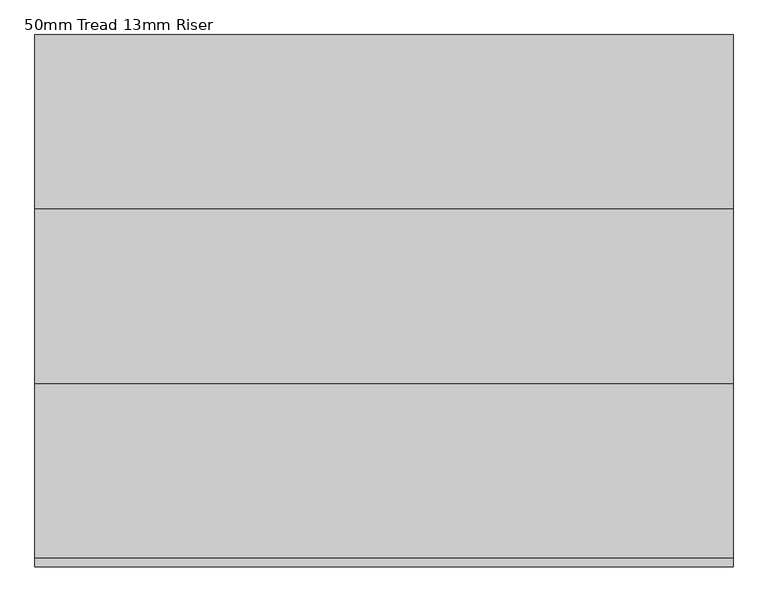
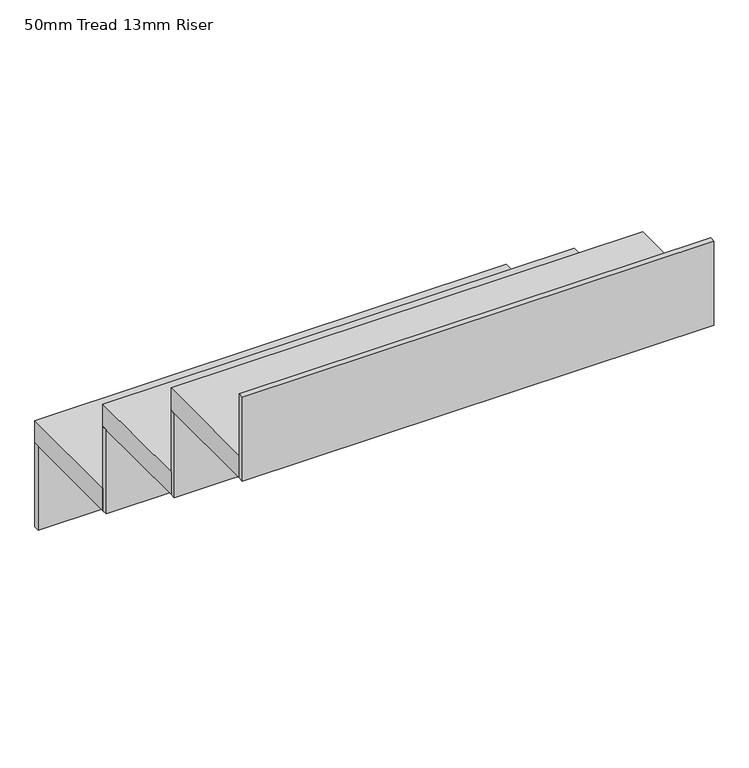
"""IFC4 building model written with IfcOpenShell, lengths in millimetres: stair flight geometry, 50mm Tread 13mm Riser."""

from ifc_helpers import new_model, si_unit, frame, origin, place, context, project, spatial, polyline, outline, extrude, source, transform, mapped, element, save


def stair_flight_50mm_tread_13mm_riser_bd8d9b2e(model_context):
    return source(origin(), model_context, "Body", "SweptSolid", [
        extrude(outline(polyline([(-10477.6052721, -2511.0618509), (-10477.6052721, -2498.5618509), (-9477.5794909, -2498.5618509), (-9477.5794909, -2511.0618509), (-10477.6052721, -2511.0618509)])), frame((0.0, 0.0, 7668.6117647), z_axis=(0.0, 0.0, 1.0), x_axis=(1.0, 0.0, 0.0)), (0.0, 0.0, 1.0), 188.2588235),
        extrude(outline(polyline([(-9477.5794909, -2748.5618509), (-10477.6052721, -2748.5618509), (-10477.6052721, -2498.5618509), (-9477.5794909, -2498.5618509), (-9477.5794909, -2748.5618509)])), frame((0.0, 0.0, 7856.8705882), z_axis=(0.0, 0.0, 1.0), x_axis=(1.0, 0.0, 0.0)), (0.0, 0.0, 1.0), 50.0),
        extrude(outline(polyline([(-10477.6052721, -2761.0618509), (-10477.6052721, -2748.5618509), (-9477.5794909, -2748.5618509), (-9477.5794909, -2761.0618509), (-10477.6052721, -2761.0618509)])), frame((0.0, 0.0, 7856.8705882), z_axis=(0.0, 0.0, 1.0), x_axis=(1.0, 0.0, 0.0)), (0.0, 0.0, 1.0), 188.2588235),
        extrude(outline(polyline([(-9477.5794909, -2998.5618509), (-10477.6052721, -2998.5618509), (-10477.6052721, -2748.5618509), (-9477.5794909, -2748.5618509), (-9477.5794909, -2998.5618509)])), frame((0.0, 0.0, 8045.1294118), z_axis=(0.0, 0.0, 1.0), x_axis=(1.0, 0.0, 0.0)), (0.0, 0.0, 1.0), 50.0),
        extrude(outline(polyline([(-10477.6052721, -3011.0618509), (-10477.6052721, -2998.5618509), (-9477.5794909, -2998.5618509), (-9477.5794909, -3011.0618509), (-10477.6052721, -3011.0618509)])), frame((0.0, 0.0, 8045.1294118), z_axis=(0.0, 0.0, 1.0), x_axis=(1.0, 0.0, 0.0)), (0.0, 0.0, 1.0), 188.2588235),
        extrude(outline(polyline([(-10477.6052721, -3261.0618509), (-10477.6052721, -3248.5618509), (-9477.5794909, -3248.5618509), (-9477.5794909, -3261.0618509), (-10477.6052721, -3261.0618509)])), frame((0.0, 0.0, 8233.3882353), z_axis=(0.0, 0.0, 1.0), x_axis=(1.0, 0.0, 0.0)), (0.0, 0.0, 1.0), 188.2588235),
        extrude(outline(polyline([(-9477.5794909, -3248.5618509), (-10477.6052721, -3248.5618509), (-10477.6052721, -2998.5618509), (-9477.5794909, -2998.5618509), (-9477.5794909, -3248.5618509)])), frame((0.0, 0.0, 8233.3882353), z_axis=(0.0, 0.0, 1.0), x_axis=(1.0, 0.0, 0.0)), (0.0, 0.0, 1.0), 50.0),
    ])


if __name__ == "__main__":
    model = new_model("IFC4")
    model_context = context("Model", 3, world=origin())
    ifc_project = project(units=[si_unit("LENGTHUNIT", "METRE", prefix="MILLI")], contexts=[model_context])
    site = spatial("IfcSite", under=ifc_project)
    building = spatial("IfcBuilding", under=site)
    placement = place(None, origin())
    stair_flight_50mm_tread_13mm_riser_shape = stair_flight_50mm_tread_13mm_riser_bd8d9b2e(model_context)
    element("IfcStairFlight", 1, ObjectType="50mm Tread 13mm Riser", at=placement, inside=building, context=model_context, shape_type="MappedRepresentation", body=[
        mapped(stair_flight_50mm_tread_13mm_riser_shape, transform((0.0, 0.0, 0.0), x_axis=(1.0, 0.0, 0.0), y_axis=(0.0, 1.0, 0.0), z_axis=(0.0, 0.0, 1.0))),
    ])
    save(model, "model.ifc")
